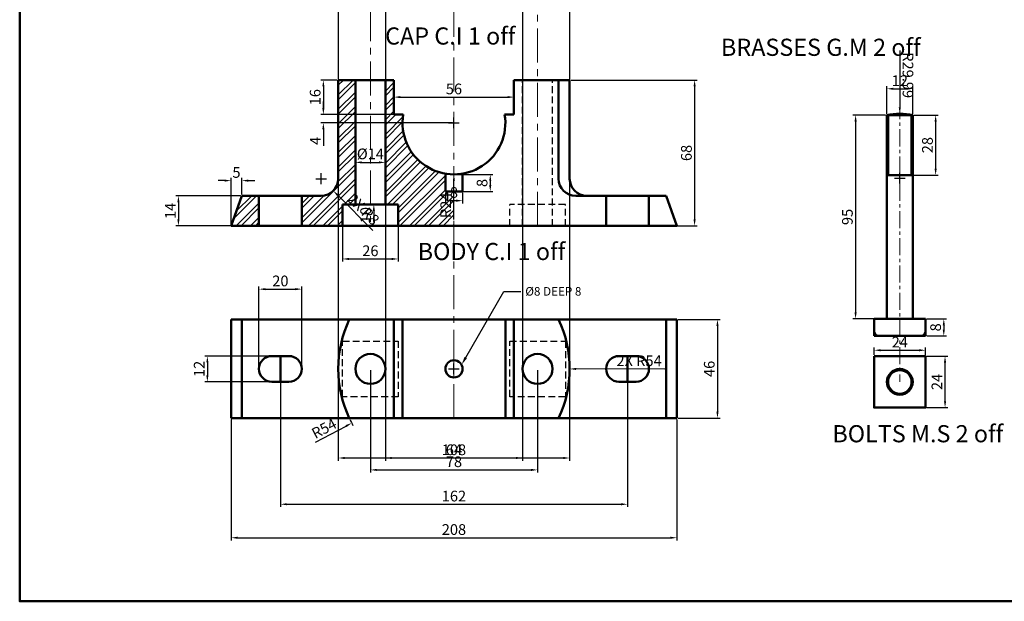
# Model space of a CAD drawing. Units: millimetres. Extents: x 6 to 817, y -61 to 407.
# Tile 1 of 3: x 6 to 466, y -61 to 210. Entities that reach past the tile are written whole.
import ezdxf
from ezdxf import colors
from ezdxf.entities.mleader import LeaderData, LeaderLine
from ezdxf.math import Vec2, Vec3

# ---------------------------------------------------------------- set-up
doc = ezdxf.new("R2010")
doc.units = ezdxf.units.MM
doc.header["$LTSCALE"] = 0.5
doc.linetypes.add('CENTER', pattern=[50.8, 31.75, -6.35, 6.35, -6.35])
doc.linetypes.add('HIDDEN', pattern=[9.525, 6.35, -3.175])
for name, color, linetype, lineweight in [('M-CNTR', 1, 'CENTER', 18), ('M-DIMS', 2, 'Continuous', 25), ('M-HATC', 8, 'Continuous', 18), ('M-HIDN', 4, 'HIDDEN', 25), ('M-OUTL', 7, 'Continuous', 50), ('M-TEXT', 3, 'Continuous', 25)]:
    doc.layers.add(name, color=color, linetype=linetype, lineweight=lineweight)
doc.styles.get("Standard").update_dxf_attribs({"font": 'arial.ttf'})
doc.dimstyles.new('ISO-25', dxfattribs={"dimtxt": 5, "dimasz": 3, "dimexe": 1.25, "dimexo": 0.625, "dimtad": 1, "dimtxsty": 'Standard', "dimcen": 2.5, "dimadec": 0, "dimazin": 0, "dimtfac": 1, "dimtofl": 0, "dimtmove": 0, "dimatfit": 3, "dimfxl": 1, "dimarcsym": 0})

# ---------------------------------------------------------------- blocks, each defined once
blk = doc.blocks.new('*D1')
at = {"layer": 'Defpoints', "color": 0, "ltscale": 0.5, "transparency": 16777216}
for p in [(105.03, 24.43), (313.03, 24.43), (313.03, -31.32)]:
    blk.add_point(p, dxfattribs=at)
at = {"layer": 'M-DIMS', "color": 0, "lineweight": -2, "ltscale": 0.5, "transparency": 16777216}
for p, q in [((105.03, 23.81), (105.03, -32.57)), ((313.03, 23.81), (313.03, -32.57)), ((108.03, -31.32), (310.03, -31.32))]:
    blk.add_line(p, q, dxfattribs=at)
at = {"layer": 'M-DIMS', "color": 0, "ltscale": 0.5, "transparency": 16777216}
for points in [[(108.03, -30.82), (108.03, -31.82), (105.03, -31.32)], [(310.03, -30.82), (310.03, -31.82), (313.03, -31.32)]]:
    blk.add_solid(points, dxfattribs=at)
at = {"layer": 'M-DIMS', "color": 0, "ltscale": 0.5, "transparency": 16777216, "insert": (209.03, -28.14), "char_height": 5, "attachment_point": 5}
blk.add_mtext('208', dxfattribs=at)
blk = doc.blocks.new('*D2')
at = {"layer": 'Defpoints', "color": 0, "ltscale": 0.5, "transparency": 16777216}
for p in [(128.03, 41.43), (290.03, 41.43), (290.03, -15.7)]:
    blk.add_point(p, dxfattribs=at)
at = {"layer": 'M-DIMS', "color": 0, "lineweight": -2, "ltscale": 0.5, "transparency": 16777216}
for p, q in [((128.03, 40.81), (128.03, -16.95)), ((290.03, 40.81), (290.03, -16.95)), ((131.03, -15.7), (287.03, -15.7))]:
    blk.add_line(p, q, dxfattribs=at)
at = {"layer": 'M-DIMS', "color": 0, "ltscale": 0.5, "transparency": 16777216}
for points in [[(131.03, -15.2), (131.03, -16.2), (128.03, -15.7)], [(287.03, -15.2), (287.03, -16.2), (290.03, -15.7)]]:
    blk.add_solid(points, dxfattribs=at)
at = {"layer": 'M-DIMS', "color": 0, "ltscale": 0.5, "transparency": 16777216, "insert": (209.03, -12.53), "char_height": 5, "attachment_point": 5}
blk.add_mtext('162', dxfattribs=at)
blk = doc.blocks.new('*D3')
at = {"layer": 'Defpoints', "color": 0, "ltscale": 0.5, "transparency": 16777216}
for p in [(170.03, 47.43), (248.03, 47.43), (248.03, 0.32)]:
    blk.add_point(p, dxfattribs=at)
at = {"layer": 'M-DIMS', "color": 0, "lineweight": -2, "ltscale": 0.5, "transparency": 16777216}
for p, q in [((170.03, 46.81), (170.03, -0.93)), ((248.03, 46.81), (248.03, -0.93)), ((173.03, 0.32), (245.03, 0.32))]:
    blk.add_line(p, q, dxfattribs=at)
at = {"layer": 'M-DIMS', "color": 0, "ltscale": 0.5, "transparency": 16777216}
for points in [[(173.03, 0.82), (173.03, -0.18), (170.03, 0.32)], [(245.03, 0.82), (245.03, -0.18), (248.03, 0.32)]]:
    blk.add_solid(points, dxfattribs=at)
at = {"layer": 'M-DIMS', "color": 0, "ltscale": 0.5, "transparency": 16777216, "insert": (209.03, 3.5), "char_height": 5, "attachment_point": 5}
blk.add_mtext('78', dxfattribs=at)
blk = doc.blocks.new('*D4')
at = {"layer": 'Defpoints', "color": 0, "ltscale": 0.5, "transparency": 16777216}
for p in [(313.03, 70.43), (313.03, 24.43), (332.01, 24.43)]:
    blk.add_point(p, dxfattribs=at)
at = {"layer": 'M-DIMS', "color": 0, "lineweight": -2, "ltscale": 0.5, "transparency": 16777216}
for p, q in [((313.66, 70.43), (333.26, 70.43)), ((332.01, 67.43), (332.01, 27.43)), ((313.66, 24.43), (333.26, 24.43))]:
    blk.add_line(p, q, dxfattribs=at)
at = {"layer": 'M-DIMS', "color": 0, "ltscale": 0.5, "transparency": 16777216}
for points in [[(331.51, 67.43), (332.51, 67.43), (332.01, 70.43)], [(331.51, 27.43), (332.51, 27.43), (332.01, 24.43)]]:
    blk.add_solid(points, dxfattribs=at)
at = {"layer": 'M-DIMS', "color": 0, "ltscale": 0.5, "transparency": 16777216, "insert": (328.83, 47.43), "char_height": 5, "attachment_point": 5, "rotation": 90}
blk.add_mtext('46', dxfattribs=at)
blk = doc.blocks.new('*D5')
at = {"layer": 'Defpoints', "color": 0, "ltscale": 0.5, "transparency": 16777216}
for p in [(209.03, 47.43), (161.31, 22.16)]:
    blk.add_point(p, dxfattribs=at)
at = {"layer": 'M-DIMS', "color": 0, "lineweight": -2, "ltscale": 0.5, "transparency": 16777216}
for p, q in [((206.53, 47.43), (211.53, 47.43)), ((209.03, 44.93), (209.03, 49.93)), ((144.36, 13.19), (158.66, 20.76))]:
    blk.add_line(p, q, dxfattribs=at)
blk.add_arc((209.03, 47.43), 54, 205.8724, 209.224, dxfattribs=at)
at = {"layer": 'M-DIMS', "color": 0, "ltscale": 0.5, "transparency": 16777216}
blk.add_solid([(158.42, 21.2), (158.89, 20.32), (161.31, 22.16)], dxfattribs=at)
at = {"layer": 'M-DIMS', "color": 0, "ltscale": 0.5, "transparency": 16777216, "insert": (148.7, 19.07), "char_height": 5, "attachment_point": 5, "rotation": 27.8977}
blk.add_mtext('R54', dxfattribs=at)
blk = doc.blocks.new('*D6')
at = {"layer": 'Defpoints', "color": 0, "ltscale": 0.5, "transparency": 16777216}
for p in [(110.03, 128.14), (80.43, 114.14), (110.03, 114.14)]:
    blk.add_point(p, dxfattribs=at)
at = {"layer": 'M-DIMS', "color": 0, "lineweight": -2, "ltscale": 0.5, "transparency": 16777216}
for p, q in [((109.41, 128.14), (79.18, 128.14)), ((80.43, 125.14), (80.43, 117.14)), ((109.41, 114.14), (79.18, 114.14))]:
    blk.add_line(p, q, dxfattribs=at)
at = {"layer": 'M-DIMS', "color": 0, "ltscale": 0.5, "transparency": 16777216}
for points in [[(79.93, 125.14), (80.93, 125.14), (80.43, 128.14)], [(79.93, 117.14), (80.93, 117.14), (80.43, 114.14)]]:
    blk.add_solid(points, dxfattribs=at)
at = {"layer": 'M-DIMS', "color": 0, "ltscale": 0.5, "transparency": 16777216, "insert": (77.29, 121.14), "char_height": 5, "attachment_point": 5, "rotation": 90}
blk.add_mtext('14', dxfattribs=at)
blk = doc.blocks.new('*D7')
at = {"layer": 'Defpoints', "color": 0, "ltscale": 0.5, "transparency": 16777216}
for p in [(110.03, 135.24), (110.03, 128.14), (105.03, 114.14)]:
    blk.add_point(p, dxfattribs=at)
at = {"layer": 'M-DIMS', "color": 0, "lineweight": -2, "ltscale": 0.5, "transparency": 16777216}
for p, q in [((102.03, 135.24), (99.03, 135.24)), ((105.03, 114.77), (105.03, 136.49)), ((110.03, 128.77), (110.03, 136.49)), ((113.03, 135.24), (116.03, 135.24))]:
    blk.add_line(p, q, dxfattribs=at)
at = {"layer": 'M-DIMS', "color": 0, "ltscale": 0.5, "transparency": 16777216}
for points in [[(102.03, 135.74), (102.03, 134.74), (105.03, 135.24)], [(113.03, 135.74), (113.03, 134.74), (110.03, 135.24)]]:
    blk.add_solid(points, dxfattribs=at)
at = {"layer": 'M-DIMS', "color": 0, "ltscale": 0.5, "transparency": 16777216, "insert": (107.53, 138.41), "char_height": 5, "attachment_point": 5}
blk.add_mtext('5', dxfattribs=at)
blk = doc.blocks.new('*D8')
at = {"layer": 'Defpoints', "color": 0, "ltscale": 0.5, "transparency": 16777216}
for p in [(157.03, 114.14), (183.03, 114.14), (183.03, 98.7)]:
    blk.add_point(p, dxfattribs=at)
at = {"layer": 'M-DIMS', "color": 0, "lineweight": -2, "ltscale": 0.5, "transparency": 16777216}
for p, q in [((157.03, 113.52), (157.03, 97.45)), ((183.03, 113.52), (183.03, 97.45)), ((160.03, 98.7), (180.03, 98.7))]:
    blk.add_line(p, q, dxfattribs=at)
at = {"layer": 'M-DIMS', "color": 0, "ltscale": 0.5, "transparency": 16777216}
for points in [[(160.03, 99.2), (160.03, 98.2), (157.03, 98.7)], [(180.03, 99.2), (180.03, 98.2), (183.03, 98.7)]]:
    blk.add_solid(points, dxfattribs=at)
at = {"layer": 'M-DIMS', "color": 0, "ltscale": 0.5, "transparency": 16777216, "insert": (170.03, 101.87), "char_height": 5, "attachment_point": 5}
blk.add_mtext('26', dxfattribs=at)
blk = doc.blocks.new('*D9')
at = {"layer": 'Defpoints', "color": 0, "ltscale": 0.5, "transparency": 16777216}
for p in [(183.03, 124.14), (171.64, 114.14), (183.03, 114.14)]:
    blk.add_point(p, dxfattribs=at)
at = {"layer": 'M-DIMS', "color": 0, "lineweight": -2, "ltscale": 0.5, "transparency": 16777216}
for p, q in [((182.41, 124.14), (170.39, 124.14)), ((171.64, 121.14), (171.64, 117.14)), ((182.41, 114.14), (170.39, 114.14))]:
    blk.add_line(p, q, dxfattribs=at)
at = {"layer": 'M-DIMS', "color": 0, "ltscale": 0.5, "transparency": 16777216}
for points in [[(171.14, 121.14), (172.14, 121.14), (171.64, 124.14)], [(171.14, 117.14), (172.14, 117.14), (171.64, 114.14)]]:
    blk.add_solid(points, dxfattribs=at)
at = {"layer": 'M-DIMS', "color": 0, "ltscale": 0.5, "transparency": 16777216, "insert": (168.46, 119.14), "char_height": 5, "attachment_point": 5, "rotation": 90}
blk.add_mtext('10', dxfattribs=at)
blk = doc.blocks.new('*D10')
at = {"layer": 'Defpoints', "color": 0, "ltscale": 0.5, "transparency": 16777216}
for p in [(205.03, 130.14), (213.03, 130.14), (213.03, 125.89)]:
    blk.add_point(p, dxfattribs=at)
at = {"layer": 'M-DIMS', "color": 0, "lineweight": -2, "ltscale": 0.5, "transparency": 16777216}
for p, q in [((205.03, 129.52), (205.03, 124.64)), ((213.03, 129.52), (213.03, 124.64)), ((208.03, 125.89), (210.03, 125.89))]:
    blk.add_line(p, q, dxfattribs=at)
at = {"layer": 'M-DIMS', "color": 0, "ltscale": 0.5, "transparency": 16777216}
for points in [[(208.03, 126.39), (208.03, 125.39), (205.03, 125.89)], [(210.03, 126.39), (210.03, 125.39), (213.03, 125.89)]]:
    blk.add_solid(points, dxfattribs=at)
at = {"layer": 'M-DIMS', "color": 0, "ltscale": 0.5, "transparency": 16777216, "insert": (209.03, 129.07), "char_height": 5, "attachment_point": 5}
blk.add_mtext('8', dxfattribs=at)
blk = doc.blocks.new('*D11')
at = {"layer": 'Defpoints', "color": 0, "ltscale": 0.5, "transparency": 16777216}
for p in [(209.03, 138.14), (209.03, 130.14), (225.97, 130.14)]:
    blk.add_point(p, dxfattribs=at)
at = {"layer": 'M-DIMS', "color": 0, "lineweight": -2, "ltscale": 0.5, "transparency": 16777216}
for p, q in [((209.66, 138.14), (227.22, 138.14)), ((225.97, 135.14), (225.97, 133.14)), ((209.66, 130.14), (227.22, 130.14))]:
    blk.add_line(p, q, dxfattribs=at)
at = {"layer": 'M-DIMS', "color": 0, "ltscale": 0.5, "transparency": 16777216}
for points in [[(225.47, 135.14), (226.47, 135.14), (225.97, 138.14)], [(225.47, 133.14), (226.47, 133.14), (225.97, 130.14)]]:
    blk.add_solid(points, dxfattribs=at)
at = {"layer": 'M-DIMS', "color": 0, "ltscale": 0.5, "transparency": 16777216, "insert": (222.79, 134.14), "char_height": 5, "attachment_point": 5, "rotation": 90}
blk.add_mtext('8', dxfattribs=at)
blk = doc.blocks.new('*D12')
at = {"layer": 'Defpoints', "color": 0, "ltscale": 0.5, "transparency": 16777216}
for p in [(155.03, 182.14), (148.08, 166.14), (181.03, 166.14)]:
    blk.add_point(p, dxfattribs=at)
at = {"layer": 'M-DIMS', "color": 0, "lineweight": -2, "ltscale": 0.5, "transparency": 16777216}
for p, q in [((154.41, 182.14), (146.83, 182.14)), ((148.08, 179.14), (148.08, 169.14)), ((180.41, 166.14), (146.83, 166.14))]:
    blk.add_line(p, q, dxfattribs=at)
at = {"layer": 'M-DIMS', "color": 0, "ltscale": 0.5, "transparency": 16777216}
for points in [[(147.58, 179.14), (148.58, 179.14), (148.08, 182.14)], [(147.58, 169.14), (148.58, 169.14), (148.08, 166.14)]]:
    blk.add_solid(points, dxfattribs=at)
at = {"layer": 'M-DIMS', "color": 0, "ltscale": 0.5, "transparency": 16777216, "insert": (144.9, 174.14), "char_height": 5, "attachment_point": 5, "rotation": 90}
blk.add_mtext('16', dxfattribs=at)
blk = doc.blocks.new('*D13')
at = {"layer": 'Defpoints', "color": 0, "ltscale": 0.5, "transparency": 16777216}
for p in [(185.37, 166.14), (148.08, 162.14), (209.03, 162.14)]:
    blk.add_point(p, dxfattribs=at)
at = {"layer": 'M-DIMS', "color": 0, "lineweight": -2, "ltscale": 0.5, "transparency": 16777216}
for p, q in [((148.08, 169.14), (148.08, 172.14)), ((184.74, 166.14), (146.83, 166.14)), ((208.41, 162.14), (146.83, 162.14)), ((148.08, 159.14), (148.08, 151.43))]:
    blk.add_line(p, q, dxfattribs=at)
at = {"layer": 'M-DIMS', "color": 0, "ltscale": 0.5, "transparency": 16777216}
for points in [[(147.58, 169.14), (148.58, 169.14), (148.08, 166.14)], [(147.58, 159.14), (148.58, 159.14), (148.08, 162.14)]]:
    blk.add_solid(points, dxfattribs=at)
at = {"layer": 'M-DIMS', "color": 0, "ltscale": 0.5, "transparency": 16777216, "insert": (144.95, 153.79), "char_height": 5, "attachment_point": 5, "rotation": 90}
blk.add_mtext('4', dxfattribs=at)
blk = doc.blocks.new('*D14')
at = {"layer": 'Defpoints', "color": 0, "ltscale": 0.5, "transparency": 16777216}
for p in [(181.03, 182.14), (237.03, 182.14), (237.03, 174.19)]:
    blk.add_point(p, dxfattribs=at)
at = {"layer": 'M-DIMS', "color": 0, "lineweight": -2, "ltscale": 0.5, "transparency": 16777216}
for p, q in [((181.03, 181.52), (181.03, 172.94)), ((237.03, 181.52), (237.03, 172.94)), ((184.03, 174.19), (234.03, 174.19))]:
    blk.add_line(p, q, dxfattribs=at)
at = {"layer": 'M-DIMS', "color": 0, "ltscale": 0.5, "transparency": 16777216}
for points in [[(184.03, 174.69), (184.03, 173.69), (181.03, 174.19)], [(234.03, 174.69), (234.03, 173.69), (237.03, 174.19)]]:
    blk.add_solid(points, dxfattribs=at)
at = {"layer": 'M-DIMS', "color": 0, "ltscale": 0.5, "transparency": 16777216, "insert": (209.03, 177.37), "char_height": 5, "attachment_point": 5}
blk.add_mtext('56', dxfattribs=at)
blk = doc.blocks.new('*D15')
at = {"layer": 'Defpoints', "color": 0, "ltscale": 0.5, "transparency": 16777216}
for p in [(163.03, 142.78), (177.03, 143.74), (177.03, 142.78)]:
    blk.add_point(p, dxfattribs=at)
at = {"layer": 'M-DIMS', "color": 0, "lineweight": -2, "ltscale": 0.5, "transparency": 16777216}
for p, q in [((163.03, 143.4), (163.03, 144.99)), ((166.03, 143.74), (174.03, 143.74)), ((177.03, 143.4), (177.03, 144.99))]:
    blk.add_line(p, q, dxfattribs=at)
at = {"layer": 'M-DIMS', "color": 0, "ltscale": 0.5, "transparency": 16777216}
for points in [[(166.03, 144.24), (166.03, 143.24), (163.03, 143.74)], [(174.03, 144.24), (174.03, 143.24), (177.03, 143.74)]]:
    blk.add_solid(points, dxfattribs=at)
at = {"layer": 'M-DIMS', "color": 0, "ltscale": 0.5, "transparency": 16777216, "insert": (170.03, 147.06), "char_height": 5, "attachment_point": 5}
blk.add_mtext('%%C14', dxfattribs=at)
blk = doc.blocks.new('*D16')
at = {"layer": 'Defpoints', "color": 0, "ltscale": 0.5, "transparency": 16777216}
for p in [(263.03, 182.14), (263.03, 114.14), (321.34, 114.14)]:
    blk.add_point(p, dxfattribs=at)
at = {"layer": 'M-DIMS', "color": 0, "lineweight": -2, "ltscale": 0.5, "transparency": 16777216}
for p, q in [((263.66, 182.14), (322.59, 182.14)), ((321.34, 179.14), (321.34, 117.14)), ((263.66, 114.14), (322.59, 114.14))]:
    blk.add_line(p, q, dxfattribs=at)
at = {"layer": 'M-DIMS', "color": 0, "ltscale": 0.5, "transparency": 16777216}
for points in [[(320.84, 179.14), (321.84, 179.14), (321.34, 182.14)], [(320.84, 117.14), (321.84, 117.14), (321.34, 114.14)]]:
    blk.add_solid(points, dxfattribs=at)
at = {"layer": 'M-DIMS', "color": 0, "ltscale": 0.5, "transparency": 16777216, "insert": (318.16, 148.14), "char_height": 5, "attachment_point": 5, "rotation": 90}
blk.add_mtext('68', dxfattribs=at)
blk = doc.blocks.new('*D17')
at = {"layer": 'Defpoints', "color": 0, "ltscale": 0.5, "transparency": 16777216}
for p in [(138.03, 84.62), (118.03, 47.43), (138.03, 47.43)]:
    blk.add_point(p, dxfattribs=at)
at = {"layer": 'M-DIMS', "color": 0, "lineweight": -2, "ltscale": 0.5, "transparency": 16777216}
for p, q in [((118.03, 48.06), (118.03, 85.87)), ((121.03, 84.62), (135.03, 84.62)), ((138.03, 48.06), (138.03, 85.87))]:
    blk.add_line(p, q, dxfattribs=at)
at = {"layer": 'M-DIMS', "color": 0, "ltscale": 0.5, "transparency": 16777216}
for points in [[(121.03, 85.12), (121.03, 84.12), (118.03, 84.62)], [(135.03, 85.12), (135.03, 84.12), (138.03, 84.62)]]:
    blk.add_solid(points, dxfattribs=at)
at = {"layer": 'M-DIMS', "color": 0, "ltscale": 0.5, "transparency": 16777216, "insert": (128.03, 87.8), "char_height": 5, "attachment_point": 5}
blk.add_mtext('20', dxfattribs=at)
blk = doc.blocks.new('*D18')
at = {"layer": 'Defpoints', "color": 0, "ltscale": 0.5, "transparency": 16777216}
for p in [(128.03, 53.43), (93.94, 41.43), (128.03, 41.43)]:
    blk.add_point(p, dxfattribs=at)
at = {"layer": 'M-DIMS', "color": 0, "lineweight": -2, "ltscale": 0.5, "transparency": 16777216}
for p, q in [((127.41, 53.43), (92.69, 53.43)), ((93.94, 50.43), (93.94, 44.43)), ((127.41, 41.43), (92.69, 41.43))]:
    blk.add_line(p, q, dxfattribs=at)
at = {"layer": 'M-DIMS', "color": 0, "ltscale": 0.5, "transparency": 16777216}
for points in [[(93.44, 50.43), (94.44, 50.43), (93.94, 53.43)], [(93.44, 44.43), (94.44, 44.43), (93.94, 41.43)]]:
    blk.add_solid(points, dxfattribs=at)
at = {"layer": 'M-DIMS', "color": 0, "ltscale": 0.5, "transparency": 16777216, "insert": (90.8, 47.43), "char_height": 5, "attachment_point": 5, "rotation": 90}
blk.add_mtext('12', dxfattribs=at)
blk = doc.blocks.new('*D41')
at = {"layer": 'Defpoints', "color": 0, "ltscale": 0.5, "transparency": 16777216}
for p in [(423.12, 178.08), (411.12, 165.8), (423.12, 165.8)]:
    blk.add_point(p, dxfattribs=at)
at = {"layer": 'M-DIMS', "color": 0, "lineweight": -2, "ltscale": 0.5, "transparency": 16777216}
for p, q in [((411.12, 166.42), (411.12, 179.33)), ((423.12, 166.42), (423.12, 179.33)), ((414.12, 178.08), (420.12, 178.08))]:
    blk.add_line(p, q, dxfattribs=at)
at = {"layer": 'M-DIMS', "color": 0, "ltscale": 0.5, "transparency": 16777216}
for points in [[(414.12, 178.58), (414.12, 177.58), (411.12, 178.08)], [(420.12, 178.58), (420.12, 177.58), (423.12, 178.08)]]:
    blk.add_solid(points, dxfattribs=at)
at = {"layer": 'M-DIMS', "color": 0, "ltscale": 0.5, "transparency": 16777216, "insert": (417.12, 181.22), "char_height": 5, "attachment_point": 5}
blk.add_mtext('12', dxfattribs=at)
blk = doc.blocks.new('*D42')
at = {"layer": 'Defpoints', "color": 0, "ltscale": 0.5, "transparency": 16777216}
for p in [(423.12, 165.8), (422.62, 137.8), (433.84, 137.8)]:
    blk.add_point(p, dxfattribs=at)
at = {"layer": 'M-DIMS', "color": 0, "lineweight": -2, "ltscale": 0.5, "transparency": 16777216}
for p, q in [((423.74, 165.8), (435.09, 165.8)), ((433.84, 162.8), (433.84, 140.8)), ((423.24, 137.8), (435.09, 137.8))]:
    blk.add_line(p, q, dxfattribs=at)
at = {"layer": 'M-DIMS', "color": 0, "ltscale": 0.5, "transparency": 16777216}
for points in [[(433.34, 162.8), (434.34, 162.8), (433.84, 165.8)], [(433.34, 140.8), (434.34, 140.8), (433.84, 137.8)]]:
    blk.add_solid(points, dxfattribs=at)
at = {"layer": 'M-DIMS', "color": 0, "ltscale": 0.5, "transparency": 16777216, "insert": (430.66, 151.8), "char_height": 5, "attachment_point": 5, "rotation": 90}
blk.add_mtext('28', dxfattribs=at)
blk = doc.blocks.new('*D43')
at = {"layer": 'Defpoints', "color": 0, "ltscale": 0.5, "transparency": 16777216}
for p in [(429.12, 70.8), (429.12, 62.8), (437.64, 62.8)]:
    blk.add_point(p, dxfattribs=at)
at = {"layer": 'M-DIMS', "color": 0, "lineweight": -2, "ltscale": 0.5, "transparency": 16777216}
for p, q in [((429.74, 70.8), (438.89, 70.8)), ((437.64, 67.8), (437.64, 65.8)), ((429.74, 62.8), (438.89, 62.8))]:
    blk.add_line(p, q, dxfattribs=at)
at = {"layer": 'M-DIMS', "color": 0, "ltscale": 0.5, "transparency": 16777216}
for points in [[(437.14, 67.8), (438.14, 67.8), (437.64, 70.8)], [(437.14, 65.8), (438.14, 65.8), (437.64, 62.8)]]:
    blk.add_solid(points, dxfattribs=at)
at = {"layer": 'M-DIMS', "color": 0, "ltscale": 0.5, "transparency": 16777216, "insert": (434.47, 66.8), "char_height": 5, "attachment_point": 5, "rotation": 90}
blk.add_mtext('8', dxfattribs=at)
blk = doc.blocks.new('*D44')
at = {"layer": 'Defpoints', "color": 0, "ltscale": 0.5, "transparency": 16777216}
for p in [(429.12, 56.13), (405.12, 53.35), (429.12, 53.35)]:
    blk.add_point(p, dxfattribs=at)
at = {"layer": 'M-DIMS', "color": 0, "lineweight": -2, "ltscale": 0.5, "transparency": 16777216}
for p, q in [((405.12, 53.98), (405.12, 57.38)), ((408.12, 56.13), (426.12, 56.13)), ((429.12, 53.98), (429.12, 57.38))]:
    blk.add_line(p, q, dxfattribs=at)
at = {"layer": 'M-DIMS', "color": 0, "ltscale": 0.5, "transparency": 16777216}
for points in [[(408.12, 56.63), (408.12, 55.63), (405.12, 56.13)], [(426.12, 56.63), (426.12, 55.63), (429.12, 56.13)]]:
    blk.add_solid(points, dxfattribs=at)
at = {"layer": 'M-DIMS', "color": 0, "ltscale": 0.5, "transparency": 16777216, "insert": (417.12, 59.27), "char_height": 5, "attachment_point": 5}
blk.add_mtext('24', dxfattribs=at)
blk = doc.blocks.new('*D45')
at = {"layer": 'Defpoints', "color": 0, "ltscale": 0.5, "transparency": 16777216}
for p in [(411.12, 165.8), (396.48, 70.8), (411.12, 70.8)]:
    blk.add_point(p, dxfattribs=at)
at = {"layer": 'M-DIMS', "color": 0, "lineweight": -2, "ltscale": 0.5, "transparency": 16777216}
for p, q in [((410.49, 165.8), (395.23, 165.8)), ((396.48, 162.8), (396.48, 73.8)), ((410.49, 70.8), (395.23, 70.8))]:
    blk.add_line(p, q, dxfattribs=at)
at = {"layer": 'M-DIMS', "color": 0, "ltscale": 0.5, "transparency": 16777216}
for points in [[(395.98, 162.8), (396.98, 162.8), (396.48, 165.8)], [(395.98, 73.8), (396.98, 73.8), (396.48, 70.8)]]:
    blk.add_solid(points, dxfattribs=at)
at = {"layer": 'M-DIMS', "color": 0, "ltscale": 0.5, "transparency": 16777216, "insert": (393.3, 118.3), "char_height": 5, "attachment_point": 5, "rotation": 90}
blk.add_mtext('95', dxfattribs=at)
blk = doc.blocks.new('SLOT-BASE')
for p, q in [((6, 12), (14, 12)), ((0, 6), (0, 6)), ((20, 6), (20, 6)), ((6, 0), (14, 0))]:
    blk.add_line(p, q)
for centre, start, end in [((6, 6), 90, 180), ((14, 6), 0, 90), ((6, 6), 180, 270), ((14, 6), 270, 0)]:
    blk.add_arc(centre, 6, start, end)
blk = doc.blocks.new('*D51')
at = {"layer": 'Defpoints', "color": 0, "ltscale": 0.5, "transparency": 16777216}
for p in [(155.03, 306.23), (263.03, 306.23), (263.03, 5.88)]:
    blk.add_point(p, dxfattribs=at)
at = {"layer": 'M-DIMS', "color": 0, "lineweight": -2, "ltscale": 0.5, "transparency": 16777216}
for p, q in [((155.03, 305.6), (155.03, 4.63)), ((263.03, 305.6), (263.03, 4.63)), ((158.03, 5.88), (260.03, 5.88))]:
    blk.add_line(p, q, dxfattribs=at)
at = {"layer": 'M-DIMS', "color": 0, "ltscale": 0.5, "transparency": 16777216}
for points in [[(158.03, 6.38), (158.03, 5.38), (155.03, 5.88)], [(260.03, 6.38), (260.03, 5.38), (263.03, 5.88)]]:
    blk.add_solid(points, dxfattribs=at)
at = {"layer": 'M-DIMS', "color": 0, "ltscale": 0.5, "transparency": 16777216, "insert": (209.03, 9.06), "char_height": 5, "attachment_point": 5}
blk.add_mtext('108', dxfattribs=at)
blk = doc.blocks.new('*D53')
at = {"layer": 'Defpoints', "color": 0, "ltscale": 0.5, "transparency": 16777216}
for p in [(177.03, 217.11), (241.03, 217.11), (241.03, 5.88)]:
    blk.add_point(p, dxfattribs=at)
at = {"layer": 'M-DIMS', "color": 0, "lineweight": -2, "ltscale": 0.5, "transparency": 16777216}
for p, q in [((177.03, 216.48), (177.03, 4.63)), ((241.03, 216.48), (241.03, 4.63)), ((180.03, 5.88), (238.03, 5.88))]:
    blk.add_line(p, q, dxfattribs=at)
at = {"layer": 'M-DIMS', "color": 0, "ltscale": 0.5, "transparency": 16777216}
for points in [[(180.03, 6.38), (180.03, 5.38), (177.03, 5.88)], [(238.03, 6.38), (238.03, 5.38), (241.03, 5.88)]]:
    blk.add_solid(points, dxfattribs=at)
at = {"layer": 'M-DIMS', "color": 0, "ltscale": 0.5, "transparency": 16777216, "insert": (209.03, 9.06), "char_height": 5, "attachment_point": 5}
blk.add_mtext('64', dxfattribs=at)
blk = doc.blocks.new('*D54')
at = {"layer": 'Defpoints', "color": 0, "ltscale": 0.5, "transparency": 16777216}
for p in [(429.12, 53.35), (438.22, 53.35), (429.12, 29.35)]:
    blk.add_point(p, dxfattribs=at)
at = {"layer": 'M-DIMS', "color": 0, "lineweight": -2, "ltscale": 0.5, "transparency": 16777216}
for p, q in [((429.74, 53.35), (439.47, 53.35)), ((438.22, 32.35), (438.22, 50.35)), ((429.74, 29.35), (439.47, 29.35))]:
    blk.add_line(p, q, dxfattribs=at)
at = {"layer": 'M-DIMS', "color": 0, "ltscale": 0.5, "transparency": 16777216}
for points in [[(437.72, 50.35), (438.72, 50.35), (438.22, 53.35)], [(437.72, 32.35), (438.72, 32.35), (438.22, 29.35)]]:
    blk.add_solid(points, dxfattribs=at)
at = {"layer": 'M-DIMS', "color": 0, "ltscale": 0.5, "transparency": 16777216, "insert": (435.08, 41.35), "char_height": 5, "attachment_point": 5, "rotation": 90}
blk.add_mtext('24', dxfattribs=at)
blk = doc.blocks.new('*D61')
at = {"layer": 'Defpoints', "color": 0, "ltscale": 0.5, "transparency": 16777216}
for p in [(209.03, 47.43), (263.03, 47.4)]:
    blk.add_point(p, dxfattribs=at)
at = {"layer": 'M-DIMS', "color": 0, "lineweight": -2, "ltscale": 0.5, "transparency": 16777216}
for p, q in [((206.53, 47.43), (211.53, 47.43)), ((209.03, 44.93), (209.03, 49.93)), ((307.43, 47.37), (266.03, 47.4))]:
    blk.add_line(p, q, dxfattribs=at)
at = {"layer": 'M-DIMS', "color": 0, "ltscale": 0.5, "transparency": 16777216}
blk.add_solid([(266.03, 47.9), (266.03, 46.9), (263.03, 47.4)], dxfattribs=at)
at = {"layer": 'M-DIMS', "color": 0, "ltscale": 0.5, "transparency": 16777216, "insert": (295.43, 50.56), "char_height": 5, "attachment_point": 5, "rotation": 359.9675}
blk.add_mtext('2X R54', dxfattribs=at)
blk = doc.blocks.new('*D62')
at = {"layer": 'Defpoints', "color": 0, "ltscale": 0.5, "transparency": 16777216}
for p in [(147.03, 136.14), (152.7, 130.5)]:
    blk.add_point(p, dxfattribs=at)
at = {"layer": 'M-DIMS', "color": 0, "lineweight": -2, "ltscale": 0.5, "transparency": 16777216}
for p, q in [((147.03, 133.64), (147.03, 138.64)), ((144.53, 136.14), (149.53, 136.14)), ((171.24, 112.05), (154.83, 128.38))]:
    blk.add_line(p, q, dxfattribs=at)
at = {"layer": 'M-DIMS', "color": 0, "ltscale": 0.5, "transparency": 16777216}
blk.add_solid([(155.18, 128.74), (154.47, 128.03), (152.7, 130.5)], dxfattribs=at)
at = {"layer": 'M-DIMS', "color": 0, "ltscale": 0.5, "transparency": 16777216, "insert": (166.34, 121.41), "char_height": 5, "attachment_point": 5, "rotation": 315.1329}
blk.add_mtext('2X R8', dxfattribs=at)
blk = doc.blocks.new('*D63')
at = {"layer": 'Defpoints', "color": 0, "ltscale": 0.5, "transparency": 16777216}
for p in [(209.03, 162.14), (209, 138.14)]:
    blk.add_point(p, dxfattribs=at)
at = {"layer": 'M-DIMS', "color": 0, "lineweight": -2, "ltscale": 0.5, "transparency": 16777216}
for p, q in [((206.53, 162.14), (211.53, 162.14)), ((209.03, 159.64), (209.03, 164.64)), ((208.97, 117.15), (209, 135.14))]:
    blk.add_line(p, q, dxfattribs=at)
at = {"layer": 'M-DIMS', "color": 0, "ltscale": 0.5, "transparency": 16777216}
blk.add_solid([(208.5, 135.14), (209.5, 135.14), (209, 138.14)], dxfattribs=at)
at = {"layer": 'M-DIMS', "color": 0, "ltscale": 0.5, "transparency": 16777216, "insert": (205.85, 123.75), "char_height": 5, "attachment_point": 5, "rotation": 89.9267}
blk.add_mtext('R24', dxfattribs=at)
blk = doc.blocks.new('*D64')
at = {"layer": 'Defpoints', "color": 0, "ltscale": 0.5, "transparency": 16777216}
for p in [(417.1, 166.4), (417.12, 136.41)]:
    blk.add_point(p, dxfattribs=at)
at = {"layer": 'M-DIMS', "color": 0, "lineweight": -2, "ltscale": 0.5, "transparency": 16777216}
for p, q in [((417.08, 195.86), (417.1, 169.4)), ((417.12, 133.91), (417.12, 138.91)), ((414.62, 136.41), (419.62, 136.41))]:
    blk.add_line(p, q, dxfattribs=at)
at = {"layer": 'M-DIMS', "color": 0, "ltscale": 0.5, "transparency": 16777216}
blk.add_solid([(417.6, 169.41), (416.6, 169.4), (417.1, 166.4)], dxfattribs=at)
at = {"layer": 'M-DIMS', "color": 0, "ltscale": 0.5, "transparency": 16777216, "insert": (420.27, 184.4), "char_height": 5, "attachment_point": 5, "rotation": 270.0337}
blk.add_mtext('R29.99', dxfattribs=at)

msp = doc.modelspace()

# ---------------------------------------------------------------- hatches: boundary and pattern name
at = {"layer": 'M-HATC', "ltscale": 0.5}
h = msp.add_hatch(dxfattribs=at)
h.set_pattern_fill('ANSI32', color=256, scale=0.5)
h.paths.add_polyline_path([(105.031, 114.143), (118.031, 114.143), (118.031, 128.143), (110.031, 128.143)])
h.paths.add_polyline_path([(147.031, 128.143), (138.031, 128.143), (138.031, 114.143), (157.031, 114.143), (157.031, 124.143), (163.031, 124.143), (163.031, 182.143), (155.031, 182.143), (155.031, 136.143, -0.4142136)])
h.paths.add_polyline_path([(183.031, 124.143), (183.031, 114.143), (209.031, 114.143), (209.031, 130.143), (205.031, 130.143), (205.031, 138.479, -0.4142136), (185.366, 166.143), (181.031, 166.143), (181.031, 182.143), (177.031, 182.143), (177.031, 124.143)])

# ---------------------------------------------------------------- linework, layer by layer
at = {"layer": 'M-CNTR'}
for p, q in [((209.031, 24.431), (209.031, 330.227)), ((170.031, 124.143), (170.031, 318.227)), ((248.031, 114.143), (248.031, 318.227))]:
    msp.add_line(p, q, dxfattribs=at)
at = {"layer": 'M-CNTR', "ltscale": 0.5}
msp.add_line((417.118, 171.864), (417.118, 41.355), dxfattribs=at)
at = {"layer": 'M-HIDN'}
for p, q in [((241.031, 114.143), (241.031, 182.143)), ((255.031, 114.143), (255.031, 182.143)), ((235.031, 114.143), (235.031, 124.143)), ((261.031, 124.143), (235.031, 124.143)), ((261.031, 114.143), (261.031, 124.143)), ((157.031, 60.431), (183.031, 60.431)), ((157.031, 34.431), (157.031, 60.431)), ((183.031, 60.431), (183.031, 34.431)), ((235.031, 60.431), (261.031, 60.431)), ((235.031, 34.431), (235.031, 60.431)), ((261.031, 60.431), (261.031, 34.431)), ((183.031, 34.431), (157.031, 34.431)), ((261.031, 34.431), (235.031, 34.431))]:
    msp.add_line(p, q, dxfattribs=at)
at = {"layer": 'M-OUTL'}
for p, q in [((155.031, 182.143), (181.031, 182.143)), ((155.031, 136.143), (155.031, 182.143)), ((163.031, 124.143), (163.031, 182.143)), ((177.031, 124.143), (177.031, 182.143)), ((181.031, 166.143), (181.031, 182.143)), ((237.031, 166.143), (237.031, 182.143)), ((237.031, 182.143), (263.031, 182.143)), ((263.031, 136.143), (263.031, 182.143)), ((105.031, 114.143), (110.031, 128.143)), ((147.031, 128.143), (110.031, 128.143)), ((118.031, 128.143), (118.031, 114.143)), ((138.031, 128.143), (138.031, 114.143)), ((157.031, 114.143), (157.031, 124.143)), ((183.031, 124.143), (157.031, 124.143)), ((183.031, 114.143), (183.031, 124.143)), ((183.031, 114.143), (183.031, 124.143)), ((308.031, 128.143), (265.888, 128.143)), ((280.031, 128.143), (280.031, 114.143)), ((300.031, 128.143), (300.031, 114.143)), ((313.031, 114.143), (308.031, 128.143)), ((105.031, 114.143), (313.031, 114.143)), ((105.031, 70.431), (313.031, 70.431)), ((105.031, 24.431), (105.031, 70.431)), ((110.031, 70.431), (110.031, 24.431)), ((308.031, 70.431), (308.031, 24.431)), ((313.031, 70.431), (313.031, 24.431)), ((128.031, 41.431), (128.031, 53.431)), ((290.031, 41.431), (290.031, 53.431)), ((313.031, 24.431), (105.031, 24.431))]:
    msp.add_line(p, q, dxfattribs=at)
at = {"layer": 'M-OUTL', "ltscale": 0.5}
for p, q in [((248.031, 182.143), (255.031, 182.143)), ((257.888, 136.143), (257.888, 182.143)), ((181.031, 166.143), (185.366, 166.143)), ((232.695, 166.143), (237.031, 166.143)), ((411.118, 165.798), (423.118, 165.798)), ((411.118, 70.798), (411.118, 165.798)), ((411.618, 137.798), (411.618, 165.896)), ((422.618, 137.798), (422.618, 165.896)), ((423.118, 165.798), (423.118, 70.798)), ((205.031, 138.479), (205.031, 130.143)), ((213.031, 130.143), (213.031, 138.479)), ((411.618, 137.798), (411.118, 138.298)), ((422.618, 137.798), (423.118, 138.298)), ((422.618, 137.798), (411.618, 137.798)), ((205.031, 130.143), (213.031, 130.143)), ((181.031, 70.431), (181.031, 24.431)), ((185.031, 70.431), (185.031, 24.431)), ((233.031, 70.431), (233.031, 24.431)), ((237.031, 70.431), (237.031, 24.431)), ((411.118, 70.798), (405.118, 70.798)), ((405.118, 70.798), (405.118, 62.798)), ((423.118, 70.798), (411.118, 70.798)), ((429.118, 70.798), (423.118, 70.798)), ((429.118, 62.798), (429.118, 70.798)), ((405.118, 62.798), (429.118, 62.798))]:
    msp.add_line(p, q, dxfattribs=at)
for points in [[(6.354, 407.228), (817.271, 407.228), (817.271, -60.955), (6.354, -60.955)], [(405.118, 53.355), (429.118, 53.355), (429.118, 29.355), (405.118, 29.355)]]:
    msp.add_lwpolyline(points, close=True, dxfattribs=at)
at = {"layer": 'M-OUTL'}
for centre, radius in [((170.031, 47.431), 7), ((209.031, 47.431), 4), ((248.031, 47.431), 7)]:
    msp.add_circle(centre, radius, dxfattribs=at)
at = {"layer": 'M-OUTL', "ltscale": 0.5}
for radius in [6, 5.5]:
    msp.add_circle((417.118, 41.355), radius, dxfattribs=at)
at = {"layer": 'M-OUTL'}
for centre, radius, start, end in [((209.031, 162.143), 24, 170.40593, 9.59407), ((147.031, 136.143), 8, 270, 0), ((265.888, 136.143), 8, 180, 270), ((271.031, 136.143), 8, 180, 270), ((209.031, 47.431), 54, 154.79071, 205.20929), ((209.031, 47.431), 54, 334.79071, 25.20929)]:
    msp.add_arc(centre, radius, start, end, dxfattribs=at)
at = {"layer": 'M-OUTL', "ltscale": 0.5}
for centre, radius, start, end in [((417.118, 136.414), 29.991, 78.45948, 101.54052), ((407.118, 64.798), 2, 180, 270), ((427.118, 64.798), 2, 270, 0)]:
    msp.add_arc(centre, radius, start, end, dxfattribs=at)

# ---------------------------------------------------------------- block references
at = {"layer": 'M-OUTL'}
for p in [(118.031, 41.431), (280.031, 41.431)]:
    msp.add_blockref('SLOT-BASE', p, dxfattribs=at)

# ---------------------------------------------------------------- texts
at = {"layer": 'M-TEXT', "ltscale": 0.5, "char_height": 8, "attachment_point": 1}
for s, width, insert in [('CAP C.I 1 off', 73.86933, (176.914, 206.69)), ('BRASSES G.M 2 off', 106.37362, (333.649, 201.421)), ('\\pxqc;BODY C.I 1 off', 77.07077, (188.009, 106.185)), ('\\pxqc;BOLTS M.S 2 off', 106.37362, (372.331, 21.199))]:
    msp.add_mtext_dynamic_manual_height_columns(s, width=width, gutter_width=12.5, heights=[0], dxfattribs=dict(at, insert=insert))

# ---------------------------------------------------------------- dimensions: what is measured, and where the dimension line sits
at = {"layer": 'M-DIMS', "ltscale": 0.5}
for base, p1, p2, override, picture, middle in [((263.031, 5.881), (155.031, 306.227), (263.031, 306.227), {"dimdec": 0, "dimlfac": 1, "dimrnd": 0, "dimzin": 0, "dimdsep": 46, "dimlunit": 2}, '*D51', (209.031, 9.059)), ((241.031, 5.881), (177.031, 217.109), (241.031, 217.109), {"dimdec": 0, "dimlfac": 1, "dimrnd": 0, "dimzin": 0, "dimdsep": 46, "dimlunit": 2}, '*D53', (209.031, 9.059)), ((423.118, 178.082), (411.118, 165.798), (423.118, 165.798), {"dimclrd": 0, "dimclre": 0, "dimclrt": 0}, '*D41', (417.118, 181.218)), ((237.031, 174.189), (181.031, 182.143), (237.031, 182.143), {"dimclrd": 0, "dimclre": 0, "dimclrt": 0}, '*D14', (209.031, 177.366)), ((110.031, 135.241), (105.031, 114.143), (110.031, 128.143), {"dimclrd": 0, "dimclre": 0, "dimclrt": 0}, '*D7', (107.531, 138.409)), ((213.031, 125.893), (205.031, 130.143), (213.031, 130.143), {"dimclrd": 0, "dimclre": 0, "dimclrt": 0}, '*D10', (209.031, 129.071)), ((183.031, 98.695), (157.031, 114.143), (183.031, 114.143), {"dimclrd": 0, "dimclre": 0, "dimclrt": 0}, '*D8', (170.031, 101.873)), ((138.031, 84.62), (118.031, 47.431), (138.031, 47.431), {"dimclrd": 0, "dimclre": 0, "dimclrt": 0}, '*D17', (128.031, 87.798)), ((429.118, 56.13), (405.118, 53.355), (429.118, 53.355), {"dimclrd": 0, "dimclre": 0, "dimclrt": 0}, '*D44', (417.118, 59.266)), ((248.031, 0.319), (170.031, 47.431), (248.031, 47.431), {"dimclrd": 0, "dimclre": 0, "dimclrt": 0}, '*D3', (209.031, 3.497)), ((290.031, -15.705), (128.031, 41.431), (290.031, 41.431), {"dimclrd": 0, "dimclre": 0, "dimclrt": 0}, '*D2', (209.031, -12.527))]:
    dim = msp.add_linear_dim(base=base, p1=p1, p2=p2, dimstyle='ISO-25', override=override, dxfattribs=at)
    dim.commit()
    dim.dimension.update_dxf_attribs({"geometry": picture, "text_midpoint": middle})
for center, mpoint, override, picture, middle in [((417.118, 136.414), (417.1, 166.405), {"dimdec": 2, "dimlfac": 1, "dimrnd": 0, "dimzin": 0, "dimdsep": 46, "dimlunit": 2}, '*D64', (417.089, 184.399)), ((209.031, 162.143), (209, 138.143), {"dimdec": 0, "dimlfac": 1, "dimrnd": 0, "dimzin": 0, "dimdsep": 46, "dimlunit": 2}, '*D63', (208.982, 123.743))]:
    dim = msp.add_radius_dim(center=center, mpoint=mpoint, dimstyle='ISO-25', override=override, dxfattribs=at)
    dim.commit()
    dim.dimension.update_dxf_attribs({"geometry": picture, "text_midpoint": middle, "dimtype": 164})
for base, p1, p2, override, picture, middle in [((148.077, 166.143), (155.031, 182.143), (181.031, 166.143), {"dimclrd": 0, "dimclre": 0, "dimclrt": 0}, '*D12', (144.9, 174.143)), ((321.339, 114.143), (263.031, 182.143), (263.031, 114.143), {"dimclrd": 0, "dimclre": 0, "dimclrt": 0}, '*D16', (318.161, 148.143)), ((148.077, 162.143), (185.366, 166.143), (209.031, 162.143), {"dimclrd": 0, "dimclre": 0, "dimclrt": 0}, '*D13', (144.952, 153.789)), ((396.482, 70.798), (411.118, 165.798), (411.118, 70.798), {"dimclrd": 0, "dimclre": 0, "dimclrt": 0}, '*D45', (393.304, 118.298)), ((433.839, 137.798), (423.118, 165.798), (422.618, 137.798), {"dimclrd": 0, "dimclre": 0, "dimclrt": 0}, '*D42', (430.661, 151.798)), ((225.97, 130.143), (209.031, 138.143), (209.031, 130.143), {"dimclrd": 0, "dimclre": 0, "dimclrt": 0}, '*D11', (222.792, 134.143)), ((80.429, 114.143), (110.031, 128.143), (110.031, 114.143), {"dimclrd": 0, "dimclre": 0, "dimclrt": 0}, '*D6', (77.294, 121.143)), ((332.009, 24.431), (313.031, 70.431), (313.031, 24.431), {"dimclrd": 0, "dimclre": 0, "dimclrt": 0}, '*D4', (328.831, 47.431)), ((437.643, 62.798), (429.118, 70.798), (429.118, 62.798), {"dimclrd": 0, "dimclre": 0, "dimclrt": 0}, '*D43', (434.465, 66.798)), ((93.939, 41.431), (128.031, 53.431), (128.031, 41.431), {"dimclrd": 0, "dimclre": 0, "dimclrt": 0}, '*D18', (90.804, 47.431)), ((438.218, 53.355), (429.118, 29.355), (429.118, 53.355), {"dimdec": 0, "dimlfac": 1, "dimrnd": 0, "dimzin": 0, "dimdsep": 46, "dimlunit": 2}, '*D54', (435.082, 41.355))]:
    dim = msp.add_linear_dim(base=base, p1=p1, p2=p2, angle=90, dimstyle='ISO-25', override=override, dxfattribs=at)
    dim.commit()
    dim.dimension.update_dxf_attribs({"geometry": picture, "text_midpoint": middle})
dim = msp.add_linear_dim(base=(177.031, 143.741), p1=(163.031, 142.779), p2=(177.031, 142.779), text='%%C<>', dimstyle='ISO-25', override={"dimclrd": 0, "dimclre": 0, "dimclrt": 0}, dxfattribs=at)
dim.commit()
dim.dimension.update_dxf_attribs({"geometry": '*D15', "text_midpoint": (170.031, 147.058)})
dim = msp.add_radius_dim(center=(147.031, 136.143), mpoint=(152.701, 130.499), text='2X <>', dimstyle='ISO-25', override={"dimdec": 0, "dimlfac": 1, "dimrnd": 0, "dimzin": 0, "dimdsep": 46, "dimlunit": 2}, dxfattribs=at)
dim.commit()
dim.dimension.update_dxf_attribs({"geometry": '*D62', "text_midpoint": (166.336, 121.411)})
dim = msp.add_linear_dim(base=(171.643, 114.143), p1=(183.031, 124.143), p2=(183.031, 114.143), angle=90, dimstyle='ISO-25', override={"dimclrd": 0, "dimclre": 0, "dimclrt": 0}, dxfattribs=at)
dim.commit()
dim.dimension.update_dxf_attribs({"geometry": '*D9', "text_midpoint": (171.643, 119.143), "dimtype": 160})
dim = msp.add_radius_dim(center=(209.031, 47.431), mpoint=(263.031, 47.4), text='2X <>', dimstyle='ISO-25', override={"dimdec": 0, "dimlfac": 1, "dimrnd": 0, "dimzin": 0, "dimdsep": 46, "dimlunit": 2}, dxfattribs=at)
dim.commit()
dim.dimension.update_dxf_attribs({"geometry": '*D61', "text_midpoint": (295.431, 47.382), "dimtype": 164})
dim = msp.add_radius_dim(center=(209.031, 47.431), mpoint=(161.306, 22.164), dimstyle='ISO-25', override={"dimclrd": 0, "dimclre": 0, "dimclrt": 0}, dxfattribs=at)
dim.commit()
dim.dimension.update_dxf_attribs({"geometry": '*D5', "text_midpoint": (148.699, 19.074)})
dim = msp.add_linear_dim(base=(313.031, -31.321), p1=(105.031, 24.431), p2=(313.031, 24.431), dimstyle='ISO-25', override={"dimclrd": 0, "dimclre": 0, "dimclrt": 0}, dxfattribs=at)
dim.commit()
dim.dimension.update_dxf_attribs({"geometry": '*D1', "text_midpoint": (209.031, -31.321), "dimtype": 160})

# ---------------------------------------------------------------- leaders
at = {"layer": 'M-TEXT', "ltscale": 0.5}
ml = msp.add_multileader_mtext('Standard', dxfattribs=at)
ml.set_content('%%C8 DEEP 8', color=256)
ml.set_leader_properties()
ml.build(insert=Vec2(0, 0))
ctx = ml.context
ctx.base_point, ctx.plane_origin = Vec3(240.317, 83.512), Vec3(212.566, 49.302)
notes = []
notes.append((ctx, [(0, (1, 1, 0), (232.317, 83.512), (1, 0), 8, [(0, [(212.566, 49.302)], 0, [])])]))
ctx.mtext.insert, ctx.mtext.flow_direction = Vec3(242.317, 85.592), 5
for ctx, leaders in notes:
    for number, flags, end, landing, length, lines in leaders:
        leader = LeaderData()
        leader.index, (leader.has_last_leader_line, leader.has_dogleg_vector, leader.attachment_direction) = number, flags
        leader.last_leader_point, leader.dogleg_vector, leader.dogleg_length = Vec3(end), Vec3(landing), length
        for number, points, colour, breaks in lines:
            line = LeaderLine()
            line.index, line.vertices, line.color, line.breaks = number, Vec3.list(points), colors.encode_raw_color(colour), breaks
            leader.lines.append(line)
        ctx.leaders.append(leader)

doc.saveas('drawing.dxf')
